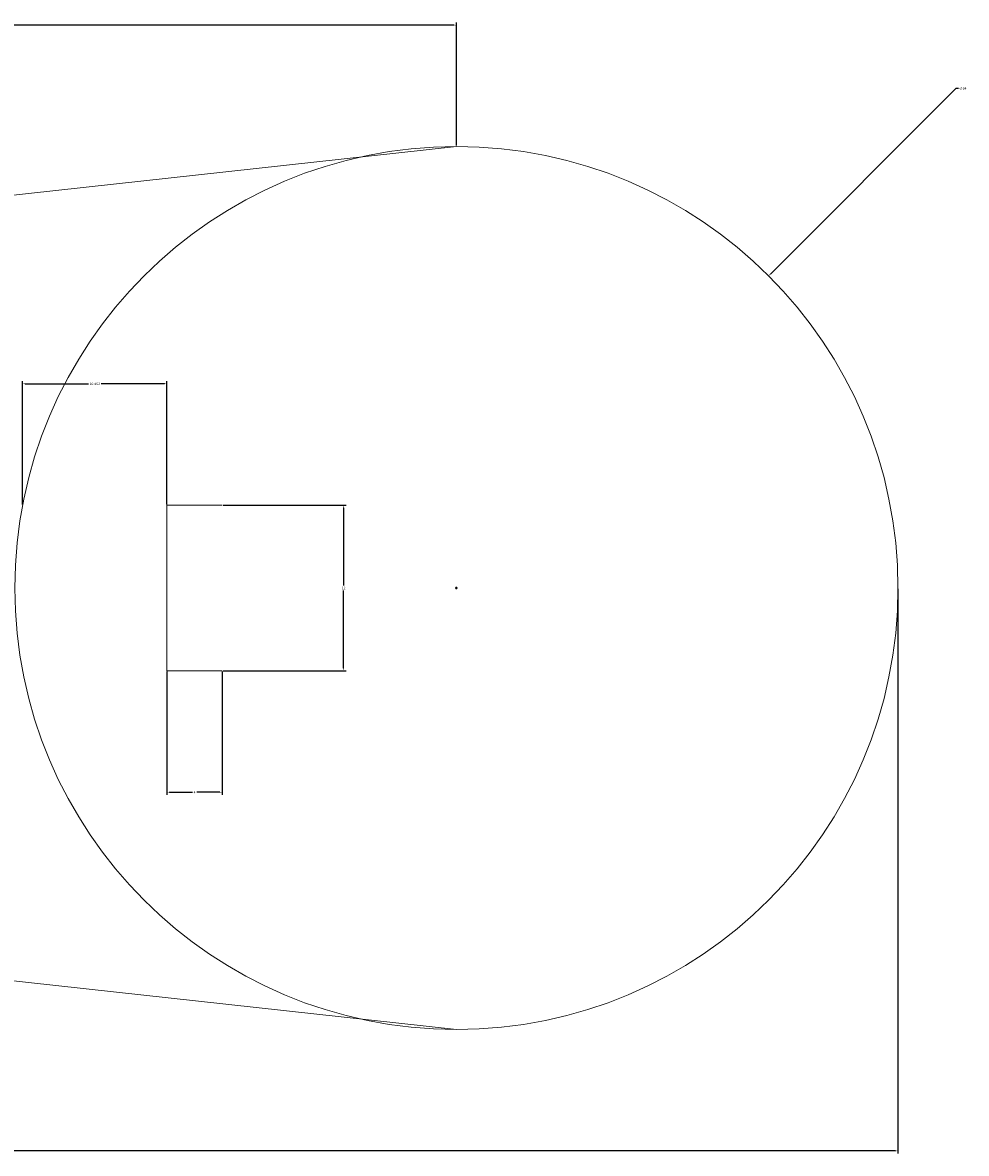
# Model space of a CAD drawing. Units: inches. Extents: x -47 to 120, y -20 to 62.
# Tile 2 of 2: x 52 to 120, y -20 to 62. Entities that reach past the tile are written whole.
import ezdxf

# ---------------------------------------------------------------- set-up
doc = ezdxf.new("R2010")
doc.units = ezdxf.units.IN
doc.header["$MEASUREMENT"] = 0
doc.layers.add('M-CONS', color=8, linetype='Continuous', lineweight=13)
doc.layers.add('M-DIMS', color=2, linetype='Continuous', lineweight=18)
doc.styles.get("Standard").update_dxf_attribs({"font": 'arial.ttf'})
doc.dimstyles.get("Standard").update_dxf_attribs({"dimtxt": 0.18, "dimasz": 0.18, "dimexe": 0.18, "dimexo": 0.0625, "dimgap": 0.09, "dimtad": 0, "dimtih": 1, "dimtoh": 1, "dimdec": 4, "dimzin": 0, "dimdsep": 46, "dimtxsty": 'Standard', "dimcen": 0.09, "dimadec": 0, "dimazin": 0, "dimtfac": 1, "dimtdec": 4, "dimtofl": 0, "dimtmove": 0, "dimatfit": 3, "dimfxl": 1, "dimtolj": 1, "dimtzin": 0, "dimarcsym": 0})

# ---------------------------------------------------------------- blocks, each defined once
blk = doc.blocks.new('*D1')
at = {"layer": 'Defpoints', "color": 0, "transparency": 16777216}
for p in [(-37.874, 20.605), (115.126, 20.605), (115.126, -20.195)]:
    blk.add_point(p, dxfattribs=at)
at = {"layer": 'M-DIMS', "color": 0, "lineweight": -2, "transparency": 16777216}
for p, q in [((-37.874, 20.542), (-37.874, -20.375)), ((115.126, 20.542), (115.126, -20.375)), ((-37.694, -20.195), (38.345, -20.195)), ((114.946, -20.195), (38.906, -20.195))]:
    blk.add_line(p, q, dxfattribs=at)
at = {"layer": 'M-DIMS', "color": 0, "transparency": 16777216}
for points in [[(-37.694, -20.165), (-37.694, -20.225), (-37.874, -20.195)], [(114.946, -20.165), (114.946, -20.225), (115.126, -20.195)]]:
    blk.add_solid(points, dxfattribs=at)
at = {"layer": 'M-DIMS', "color": 0, "transparency": 16777216, "insert": (38.626, -20.195), "char_height": 0.18, "attachment_point": 5}
blk.add_mtext('\\A1;153', dxfattribs=at)
blk = doc.blocks.new('*D2')
at = {"layer": 'Defpoints', "color": 0, "transparency": 16777216}
for p in [(83.126, 61.405), (83.126, 52.605), (-16.874, 41.605)]:
    blk.add_point(p, dxfattribs=at)
at = {"layer": 'M-DIMS', "color": 0, "lineweight": -2, "transparency": 16777216}
for p, q in [((-16.874, 41.667), (-16.874, 61.585)), ((83.126, 52.667), (83.126, 61.585)), ((-16.694, 61.405), (32.846, 61.405)), ((82.946, 61.405), (33.406, 61.405))]:
    blk.add_line(p, q, dxfattribs=at)
at = {"layer": 'M-DIMS', "color": 0, "transparency": 16777216}
for points in [[(-16.694, 61.435), (-16.694, 61.375), (-16.874, 61.405)], [(82.946, 61.435), (82.946, 61.375), (83.126, 61.405)]]:
    blk.add_solid(points, dxfattribs=at)
at = {"layer": 'M-DIMS', "color": 0, "transparency": 16777216, "insert": (33.126, 61.405), "char_height": 0.18, "attachment_point": 5}
blk.add_mtext('\\A1;100', dxfattribs=at)
blk = doc.blocks.new('*D3')
at = {"layer": 'Defpoints', "color": 0, "transparency": 16777216}
for p in [(66.155, 26.605), (66.155, 14.605), (74.955, 14.605)]:
    blk.add_point(p, dxfattribs=at)
at = {"layer": 'M-DIMS', "color": 0, "lineweight": -2, "transparency": 16777216}
for p, q in [((66.218, 26.605), (75.135, 26.605)), ((74.955, 26.425), (74.955, 20.785)), ((74.955, 14.785), (74.955, 20.424)), ((66.218, 14.605), (75.135, 14.605))]:
    blk.add_line(p, q, dxfattribs=at)
at = {"layer": 'M-DIMS', "color": 0, "transparency": 16777216}
for points in [[(74.925, 26.425), (74.985, 26.425), (74.955, 26.605)], [(74.925, 14.785), (74.985, 14.785), (74.955, 14.605)]]:
    blk.add_solid(points, dxfattribs=at)
at = {"layer": 'M-DIMS', "color": 0, "transparency": 16777216, "insert": (74.955, 20.605), "char_height": 0.18, "attachment_point": 5}
blk.add_mtext('\\A1;12', dxfattribs=at)
blk = doc.blocks.new('*D4')
at = {"layer": 'Defpoints', "color": 0, "transparency": 16777216}
for p in [(62.155, 35.405), (51.693, 26.605), (62.155, 26.605)]:
    blk.add_point(p, dxfattribs=at)
at = {"layer": 'M-DIMS', "color": 0, "lineweight": -2, "transparency": 16777216}
for p, q in [((51.693, 26.667), (51.693, 35.585)), ((51.873, 35.405), (56.47, 35.405)), ((61.975, 35.405), (57.378, 35.405)), ((62.155, 26.667), (62.155, 35.585))]:
    blk.add_line(p, q, dxfattribs=at)
at = {"layer": 'M-DIMS', "color": 0, "transparency": 16777216}
for points in [[(51.873, 35.435), (51.873, 35.375), (51.693, 35.405)], [(61.975, 35.435), (61.975, 35.375), (62.155, 35.405)]]:
    blk.add_solid(points, dxfattribs=at)
at = {"layer": 'M-DIMS', "color": 0, "transparency": 16777216, "insert": (56.924, 35.405), "char_height": 0.18, "attachment_point": 5}
blk.add_mtext('\\A1;10.462', dxfattribs=at)
blk = doc.blocks.new('*D5')
at = {"layer": 'Defpoints', "color": 0, "transparency": 16777216}
for p in [(62.155, 14.605), (66.155, 14.605), (62.155, 5.805)]:
    blk.add_point(p, dxfattribs=at)
at = {"layer": 'M-DIMS', "color": 0, "lineweight": -2, "transparency": 16777216}
for p, q in [((62.155, 14.542), (62.155, 5.625)), ((66.155, 14.542), (66.155, 5.625)), ((62.335, 5.805), (64.003, 5.805)), ((65.975, 5.805), (64.307, 5.805))]:
    blk.add_line(p, q, dxfattribs=at)
at = {"layer": 'M-DIMS', "color": 0, "transparency": 16777216}
for points in [[(62.335, 5.835), (62.335, 5.775), (62.155, 5.805)], [(65.975, 5.835), (65.975, 5.775), (66.155, 5.805)]]:
    blk.add_solid(points, dxfattribs=at)
at = {"layer": 'M-DIMS', "color": 0, "transparency": 16777216, "insert": (64.155, 5.805), "char_height": 0.18, "attachment_point": 5}
blk.add_mtext('\\A1;4', dxfattribs=at)
blk = doc.blocks.new('*D7')
at = {"layer": 'Defpoints', "color": 0, "transparency": 16777216}
for p in [(105.753, 43.233), (60.499, -2.023)]:
    blk.add_point(p, dxfattribs=at)
at = {"layer": 'M-DIMS', "color": 0, "lineweight": -2, "transparency": 16777216}
for p, q in [((119.329, 56.809), (105.88, 43.36)), ((119.509, 56.809), (119.329, 56.809)), ((83.036, 20.605), (83.216, 20.605)), ((83.126, 20.515), (83.126, 20.695))]:
    blk.add_line(p, q, dxfattribs=at)
at = {"layer": 'M-DIMS', "color": 0, "transparency": 16777216}
blk.add_solid([(105.859, 43.381), (105.901, 43.339), (105.753, 43.233)], dxfattribs=at)
at = {"layer": 'M-DIMS', "color": 0, "transparency": 16777216, "insert": (119.825, 56.809), "char_height": 0.18, "attachment_point": 5}
blk.add_mtext('\\A1;∅64', dxfattribs=at)

msp = doc.modelspace()

# ---------------------------------------------------------------- linework, layer by layer
at = {"layer": 'M-CONS'}
for p, q in [((-16.8743, 41.6047), (83.1257, 52.6047)), ((62.1552, 26.6047), (62.1552, 14.6047)), ((62.1552, 26.6047), (66.1552, 26.6047)), ((62.1552, 14.6047), (66.1552, 14.6047)), ((-16.8743, -0.3953), (83.1257, -11.3953))]:
    msp.add_line(p, q, dxfattribs=at)
msp.add_circle((83.1257, 20.6047), 32, dxfattribs=at)

# ---------------------------------------------------------------- dimensions: what is measured, and where the dimension line sits
at = {"layer": 'M-DIMS'}
for base, p1, p2, picture, middle in [((83.1257, 61.4047), (-16.8743, 41.6047), (83.1257, 52.6047), '*D2', (33.1257, 61.4047)), ((115.1257, -20.1953), (-37.8743, 20.6047), (115.1257, 20.6047), '*D1', (38.6257, -20.1953))]:
    dim = msp.add_linear_dim(base=base, p1=p1, p2=p2, dimstyle='Standard', override={"dimdec": 0, "dimlfac": 1, "dimrnd": 0, "dimzin": 0, "dimdsep": 46, "dimlunit": 2}, dxfattribs=at)
    dim.commit()
    dim.dimension.update_dxf_attribs({"geometry": picture, "text_midpoint": middle})
dim = msp.add_diameter_dim_2p(p1=(60.4988, -2.0232), p2=(105.7527, 43.2326), dimstyle='Standard', override={"dimdec": 0, "dimlfac": 1, "dimrnd": 0, "dimzin": 0, "dimdsep": 46, "dimlunit": 2}, dxfattribs=at)
dim.commit()
dim.dimension.update_dxf_attribs({"geometry": '*D7', "text_midpoint": (119.8253, 56.8094), "dimtype": 163})
for base, p1, p2, angle, override, picture, middle in [((62.1552, 35.4047), (51.6933, 26.6047), (62.1552, 26.6047), 0, {"dimdec": 3, "dimlfac": 1, "dimrnd": 0, "dimzin": 0, "dimdsep": 46, "dimlunit": 2}, '*D4', (56.9242, 35.4047)), ((74.9552, 14.6047), (66.1552, 26.6047), (66.1552, 14.6047), 270, {"dimdec": 0, "dimlfac": 1, "dimrnd": 0, "dimzin": 0, "dimdsep": 46, "dimlunit": 2}, '*D3', (74.9552, 20.6047)), ((62.1552, 5.8047), (66.1552, 14.6047), (62.1552, 14.6047), 180, {"dimdec": 0, "dimlfac": 1, "dimrnd": 0, "dimzin": 0, "dimdsep": 46, "dimlunit": 2}, '*D5', (64.1552, 5.8047))]:
    dim = msp.add_linear_dim(base=base, p1=p1, p2=p2, angle=angle, dimstyle='Standard', override=override, dxfattribs=at)
    dim.commit()
    dim.dimension.update_dxf_attribs({"geometry": picture, "text_midpoint": middle})

doc.saveas('drawing.dxf')
